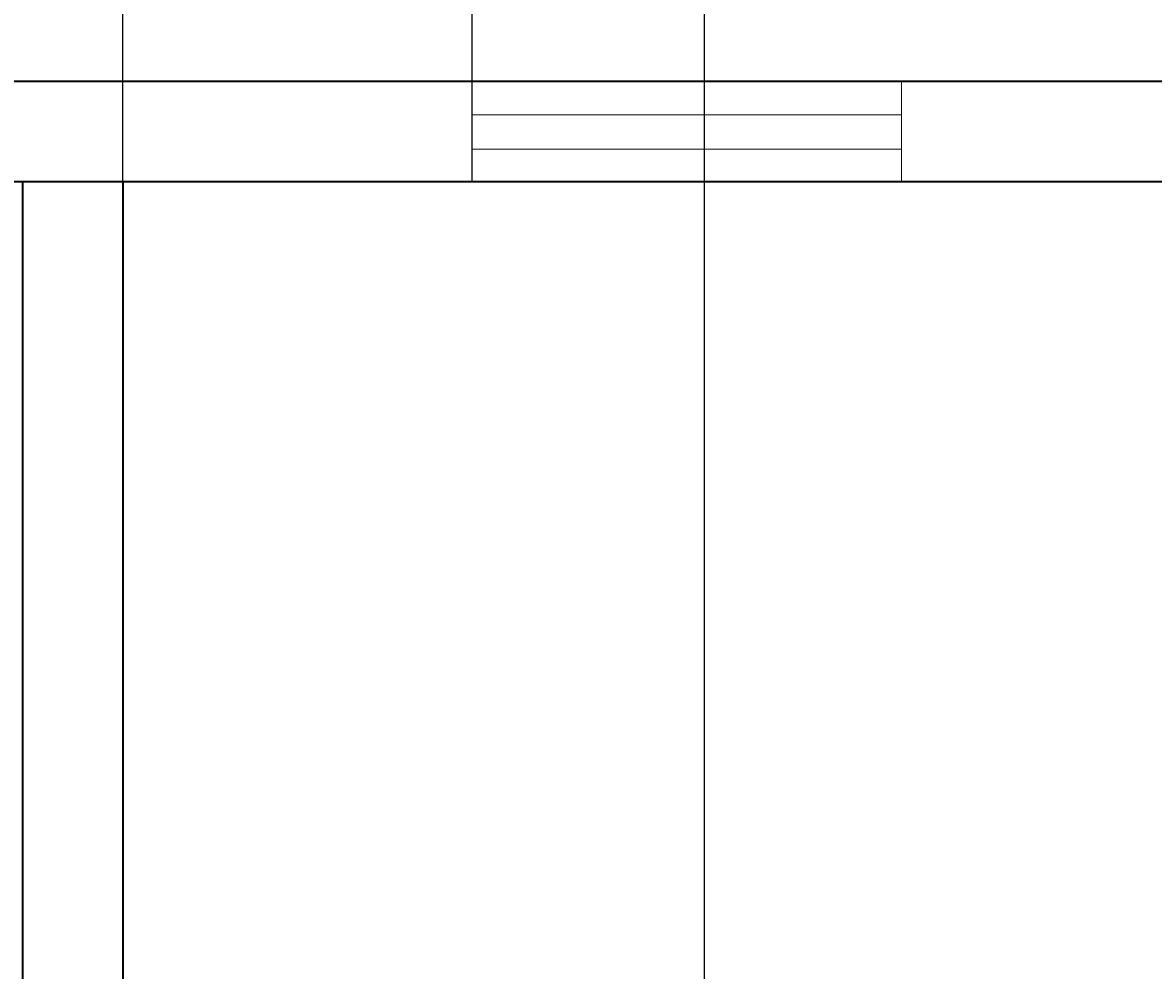
# Model space of a CAD drawing. Units: inches. Extents: x 867 to 1667, y -234 to 788.
# Tile 39 of 42: x 1395 to 1497, y 487 to 572. Entities that reach past the tile are written whole.
import ezdxf

# ---------------------------------------------------------------- set-up
doc = ezdxf.new("R2010")
doc.units = ezdxf.units.IN
doc.header["$MEASUREMENT"] = 0
for name, color, linetype, lineweight in [('A-ANNO-DIMS', 2, 'Continuous', 18), ('A-Glaz', 92, 'Continuous', 18), ('A-Wall', 7, 'Continuous', 35)]:
    doc.layers.add(name, color=color, linetype=linetype, lineweight=lineweight)
doc.styles.get("Standard").update_dxf_attribs({"font": 'arial.ttf'})
doc.dimstyles.get("Standard").update_dxf_attribs({"dimtxt": 0.6875, "dimasz": 0.18, "dimexe": 0.18, "dimexo": 0.0625, "dimgap": 0.09, "dimtad": 0, "dimdec": 4, "dimzin": 0, "dimdsep": 46, "dimlunit": 4, "dimtxsty": 'Standard', "dimcen": 0.09, "dimadec": 0, "dimazin": 0, "dimtfac": 1, "dimtdec": 4, "dimtofl": 0, "dimtmove": 0, "dimatfit": 3, "dimfxl": 1, "dimtolj": 1, "dimtzin": 0, "dimarcsym": 0})

# ---------------------------------------------------------------- blocks, each defined once
blk = doc.blocks.new('WIN-38_58IN')
for p, q in [((0, 9), (0, 0)), ((38.58, 0), (38.58, 9)), ((0, 6), (38.58, 6)), ((0, 2.92), (38.58, 2.92)), ((0, 0), (38.58, 0))]:
    blk.add_line(p, q)
blk = doc.blocks.new('*D31')
at = {"layer": 'A-ANNO-DIMS', "color": 0, "lineweight": -2, "transparency": 16777216}
for p, q in [((1070.89, 566.68), (1070.89, 787.75)), ((1071.07, 787.57), (1304.02, 787.57)), ((1538.71, 787.57), (1305.75, 787.57)), ((1538.89, 566.68), (1538.89, 787.75))]:
    blk.add_line(p, q, dxfattribs=at)
at = {"layer": 'A-ANNO-DIMS', "color": 0, "transparency": 16777216}
for points in [[(1071.07, 787.6), (1071.07, 787.54), (1070.89, 787.57)], [(1538.71, 787.6), (1538.71, 787.54), (1538.89, 787.57)]]:
    blk.add_solid(points, dxfattribs=at)
at = {"layer": 'Defpoints', "color": 0, "transparency": 16777216}
for p in [(1538.89, 787.57), (1070.89, 566.62), (1538.89, 566.62)]:
    blk.add_point(p, dxfattribs=at)
at = {"layer": 'A-ANNO-DIMS', "color": 0, "transparency": 16777216, "insert": (1304.89, 787.57), "char_height": 0.688, "attachment_point": 5}
blk.add_mtext('\\A1;468', dxfattribs=at)
blk = doc.blocks.new('*D53')
at = {"layer": 'A-ANNO-DIMS', "color": 0, "lineweight": -2, "transparency": 16777216}
for p, q in [((1403.89, 557.68), (1403.89, 787.75)), ((1404.07, 787.57), (1418.33, 787.57)), ((1435.1, 787.57), (1420.83, 787.57)), ((1435.28, 557.68), (1435.28, 787.75))]:
    blk.add_line(p, q, dxfattribs=at)
at = {"layer": 'A-ANNO-DIMS', "color": 0, "transparency": 16777216}
for points in [[(1404.07, 787.6), (1404.07, 787.54), (1403.89, 787.57)], [(1435.1, 787.6), (1435.1, 787.54), (1435.28, 787.57)]]:
    blk.add_solid(points, dxfattribs=at)
at = {"layer": 'Defpoints', "color": 0, "transparency": 16777216}
for p in [(1403.89, 787.57), (1403.89, 557.62), (1435.28, 557.62)]:
    blk.add_point(p, dxfattribs=at)
at = {"layer": 'A-ANNO-DIMS', "color": 0, "transparency": 16777216, "insert": (1419.58, 787.57), "char_height": 0.688, "attachment_point": 5}
blk.add_mtext('\\A1;31.39', dxfattribs=at)
blk = doc.blocks.new('*D54')
at = {"layer": 'A-ANNO-DIMS', "color": 0, "lineweight": -2, "transparency": 16777216}
for p, q in [((1403.89, 413.68), (1403.89, 787.75)), ((1404.07, 787.57), (1428.77, 787.57)), ((1455.97, 787.57), (1431.27, 787.57)), ((1456.15, 413.68), (1456.15, 787.75))]:
    blk.add_line(p, q, dxfattribs=at)
at = {"layer": 'A-ANNO-DIMS', "color": 0, "transparency": 16777216}
for points in [[(1404.07, 787.6), (1404.07, 787.54), (1403.89, 787.57)], [(1455.97, 787.6), (1455.97, 787.54), (1456.15, 787.57)]]:
    blk.add_solid(points, dxfattribs=at)
at = {"layer": 'Defpoints', "color": 0, "transparency": 16777216}
for p in [(1456.15, 787.57), (1403.89, 413.62), (1456.15, 413.62)]:
    blk.add_point(p, dxfattribs=at)
at = {"layer": 'A-ANNO-DIMS', "color": 0, "transparency": 16777216, "insert": (1430.02, 787.57), "char_height": 0.688, "attachment_point": 5}
blk.add_mtext('\\A1;52.27', dxfattribs=at)

msp = doc.modelspace()

# ---------------------------------------------------------------- linework, layer by layer
at = {"layer": 'A-Wall'}
for p, q in [((1538.8866, 566.617), (1070.8866, 566.617)), ((1538.8866, 557.617), (1070.8866, 557.617)), ((1394.8866, 557.617), (1394.8866, 449.617)), ((1403.8866, 557.617), (1403.8866, 449.617))]:
    msp.add_line(p, q, dxfattribs=at)

# ---------------------------------------------------------------- block references
at = {"layer": 'A-Glaz'}
msp.add_blockref('WIN-38_58IN', (1435.2759, 557.617), dxfattribs=at)

# ---------------------------------------------------------------- dimensions: what is measured, and where the dimension line sits
at = {"layer": 'A-ANNO-DIMS'}
for base, p1, p2, override, picture, middle in [((1538.8866, 787.567), (1070.8866, 566.617), (1538.8866, 566.617), {"dimdec": 0, "dimlfac": 1, "dimrnd": 0, "dimzin": 0, "dimdsep": 46, "dimlunit": 2}, '*D31', (1304.8866, 787.567)), ((1403.8866, 787.567), (1435.2754, 557.617), (1403.8866, 557.617), {"dimdec": 2, "dimlfac": 1, "dimrnd": 0, "dimzin": 0, "dimdsep": 46, "dimlunit": 2}, '*D53', (1419.581, 787.567)), ((1456.1541, 787.567), (1403.8866, 413.617), (1456.1541, 413.617), {"dimdec": 2, "dimlfac": 1, "dimrnd": 0, "dimzin": 0, "dimdsep": 46, "dimlunit": 2}, '*D54', (1430.0204, 787.567))]:
    dim = msp.add_linear_dim(base=base, p1=p1, p2=p2, dimstyle='Standard', override=override, dxfattribs=at)
    dim.commit()
    dim.dimension.update_dxf_attribs({"geometry": picture, "text_midpoint": middle})

doc.saveas('drawing.dxf')
